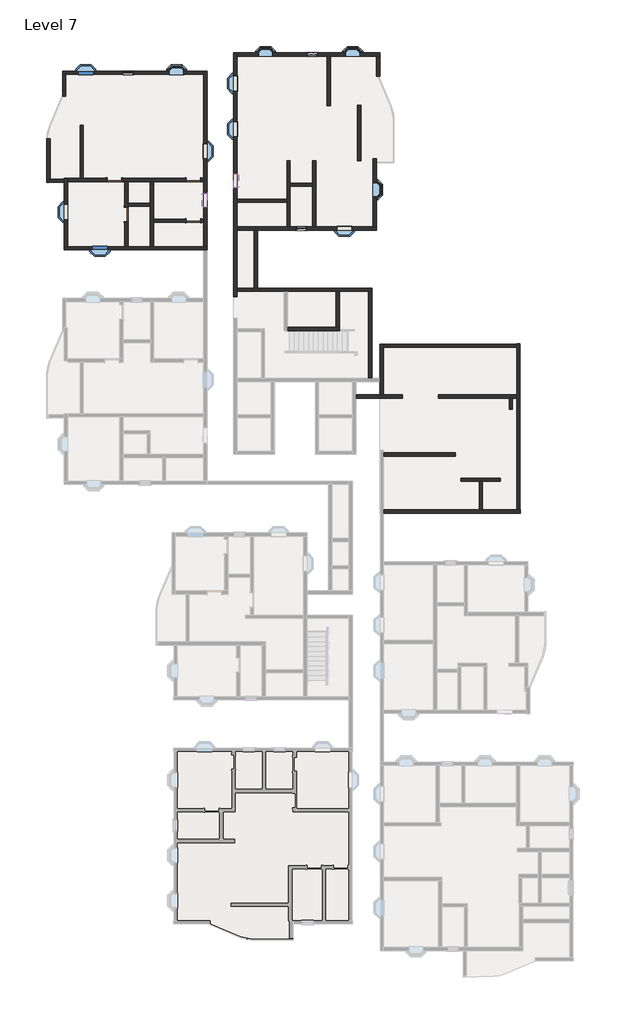
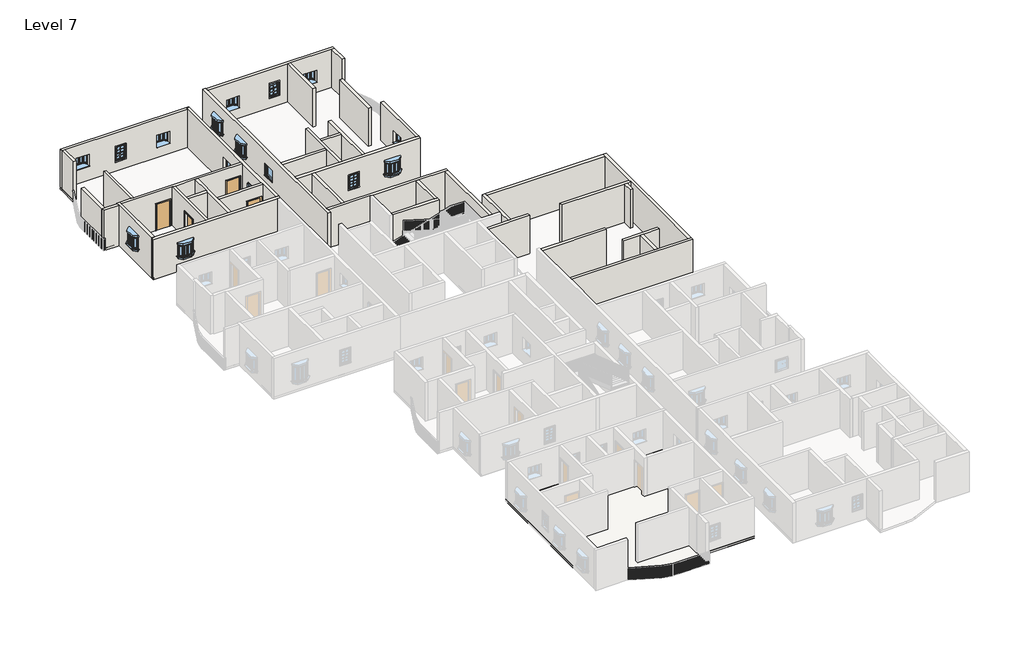
# One storey, part 4 of 14: 39 walls, 16 windows, 4 doors, 2 roofs.
"""IFC4 building model written with IfcOpenShell, lengths in millimetres."""

from ifc_helpers import new_model, si_unit, point, frame, frame_2d, origin, place, context, project, spatial, polyline, circle_curve, trimmed, segment, composite_curve, outline, extrude, faceted_brep, transform, mapped, element, save
from components import door_719f80de, window_910x910mm_67ef725a, window_8debb0fa, windows_sgl_w_glazing_bars_910x910mm_256712d0

model = new_model("IFC4")

# Units and contexts
model_context = context("Model", 3, world=origin())
ifc_project = project(units=[si_unit("LENGTHUNIT", "METRE", prefix="MILLI")], contexts=[model_context])

# Site, building, storey
site = spatial("IfcSite", under=ifc_project)
building = spatial("IfcBuilding", under=site)
storey = spatial("IfcBuildingStorey", under=building, Name="Level 7", Elevation=18288.0)

# Doors
placement = place(None, origin())
door_shape = door_719f80de(model_context)
element("IfcDoor", 1, ObjectType="Single-Flush : 36\" x 84\"", at=placement, inside=storey, context=model_context, shape_type="MappedRepresentation", body=[
    mapped(door_shape, transform((-16068.1391351, 22048.4083494, 18288.0), x_axis=(1.0, 0.0, 0.0), y_axis=(0.0, 1.0, 0.0), z_axis=(0.0, 0.0, 1.0))),
])
element("IfcDoor", 2, ObjectType="Single-Flush : 36\" x 84\"", at=placement, inside=storey, context=model_context, shape_type="MappedRepresentation", body=[
    mapped(door_shape, transform((-15306.1391351, 19864.0083494, 18288.0), x_axis=(0.0, 1.0, 0.0), y_axis=(-1.0, 0.0, 0.0), z_axis=(0.0, 0.0, 1.0))),
])
element("IfcDoor", 3, ObjectType="Single-Flush : 36\" x 84\"", at=placement, inside=storey, context=model_context, shape_type="MappedRepresentation", body=[
    mapped(door_shape, transform((-11057.9891351, 19470.3083494, 18288.0), x_axis=(1.0, 0.0, 0.0), y_axis=(0.0, 1.0, 0.0), z_axis=(0.0, 0.0, 1.0))),
])
element("IfcDoor", 4, ObjectType="Single-Flush : 36\" x 84\"", at=placement, inside=storey, context=model_context, shape_type="MappedRepresentation", body=[
    mapped(door_shape, transform((-11057.9891351, 22048.4083494, 18288.0), x_axis=(1.0, 0.0, 0.0), y_axis=(0.0, 1.0, 0.0), z_axis=(0.0, 0.0, 1.0))),
])

# Roofs
element("IfcRoof", 5, ObjectType="Generic - 12\"", at=placement, inside=storey, context=model_context, shape_type="SweptSolid", body=[
    extrude(outline(composite_curve([segment(polyline([(-10024.8708389, -25100.3416506), (-12290.487215, -25100.3416506), (-12290.487215, -13962.4416506), (-986.8891351, -13962.4416506), (-986.8891351, -25100.3416506), (-4746.0891351, -25100.3416506), (-4746.0891351, -26090.9416506), (-7315.6413127, -26090.9416506)]), True, "CONTINUOUS"), segment(trimmed(circle_curve(frame_2d((-7315.6413127, -24160.5416506)), 1930.4), [point((-7315.6413127, -26090.9416506))], [point((-8075.5356374, -25935.0851906))], False, "CARTESIAN"), True, "CONTINUOUS"), segment(polyline([(-8075.5356374, -25935.0851906), (-10024.8708389, -25100.3416506)]), True, "CONTINUOUS")], self_intersect=False)), frame((0.0, 0.0, 18288.0), z_axis=(0.0, 0.0, 1.0), x_axis=(1.0, 0.0, 0.0)), (0.0, 0.0, 1.0), 152.4),
])
element("IfcRoof", 6, ObjectType="Generic - 12\"", at=placement, inside=storey, context=model_context, shape_type="SweptSolid", body=[
    extrude(outline(composite_curve([segment(polyline([(-10024.8708389, -25100.3416506), (-12290.487215, -25100.3416506), (-12290.487215, -13962.4416506), (-986.8891351, -13962.4416506), (-986.8891351, -25100.3416506), (-4746.0891351, -25100.3416506), (-4746.0891351, -26090.9416506), (-7315.6413127, -26090.9416506)]), True, "CONTINUOUS"), segment(trimmed(circle_curve(frame_2d((-7315.6413127, -24160.5416506)), 1930.4), [point((-7315.6413127, -26090.9416506))], [point((-8075.5356374, -25935.0851906))], False, "CARTESIAN"), True, "CONTINUOUS"), segment(polyline([(-8075.5356374, -25935.0851906), (-10024.8708389, -25100.3416506)]), True, "CONTINUOUS")], self_intersect=False)), frame((0.0, 0.0, 18288.0), z_axis=(0.0, 0.0, 1.0), x_axis=(1.0, 0.0, 0.0)), (0.0, 0.0, 1.0), 152.4),
])

# Walls
element("IfcWall", 7, ObjectType="4.5\" p", at=placement, inside=storey, context=model_context, shape_type="Brep", body=[
    faceted_brep([(-10600.7891351, 21946.8083494, 20421.6), (-10600.7891351, 21946.8083494, 18288.0), (-10397.5891351, 21946.8083494, 18288.0), (-10397.5891351, 21946.8083494, 21336.0), (-13578.9391351, 21946.8083494, 21336.0), (-13782.1391351, 21946.8083494, 21336.0), (-15204.5391351, 21946.8083494, 21336.0), (-15407.7391351, 21946.8083494, 21336.0), (-19033.5891351, 21946.8083494, 21336.0), (-19033.5891351, 21946.8083494, 18288.0), (-16525.3391351, 21946.8083494, 18288.0), (-16525.3391351, 21946.8083494, 20421.6), (-15610.9391351, 21946.8083494, 20421.6), (-15610.9391351, 21946.8083494, 18288.0), (-15407.7391351, 21946.8083494, 18288.0), (-15204.5391351, 21946.8083494, 18288.0), (-13782.1391351, 21946.8083494, 18288.0), (-13578.9391351, 21946.8083494, 18288.0), (-11515.1891351, 21946.8083494, 18288.0), (-11515.1891351, 21946.8083494, 20421.6), (-10397.5891351, 22150.0083494, 18288.0), (-10600.7891351, 22150.0083494, 18288.0), (-10600.7891351, 22150.0083494, 20421.6), (-11515.1891351, 22150.0083494, 20421.6), (-11515.1891351, 22150.0083494, 18288.0), (-15610.9391351, 22150.0083494, 18288.0), (-15610.9391351, 22150.0083494, 20421.6), (-16525.3391351, 22150.0083494, 20421.6), (-16525.3391351, 22150.0083494, 18288.0), (-18042.9891351, 22150.0083494, 18288.0), (-18246.1891351, 22150.0083494, 18288.0), (-19033.5891351, 22150.0083494, 18288.0), (-19033.5891351, 22150.0083494, 21336.0), (-18246.1891351, 22150.0083494, 21336.0), (-18042.9891351, 22150.0083494, 21336.0), (-10397.5891351, 22150.0083494, 21336.0)], [[[0, 1, 2, 3, 4, 5, 6, 7, 8, 9, 10, 11, 12, 13, 14, 15, 16, 17, 18, 19]], [[20, 21, 22, 23, 24, 25, 26, 27, 28, 29, 30, 31, 32, 33, 34, 35]], [[10, 9, 31, 30, 29, 28]], [[2, 1, 21, 20]], [[18, 17, 16, 15, 14, 13, 25, 24]], [[8, 7, 6, 5, 4, 3, 35, 34, 33, 32]], [[9, 8, 32, 31]], [[3, 2, 20, 35]], [[26, 25, 13, 12]], [[27, 26, 12, 11]], [[28, 27, 11, 10]], [[22, 21, 1, 0]], [[23, 22, 0, 19]], [[24, 23, 19, 18]]]),
])
element("IfcWall", 8, ObjectType="4.5\" p", at=placement, inside=storey, context=model_context, shape_type="Brep", body=[
    faceted_brep([(-15407.7391351, 21946.8083494, 18288.0), (-15407.7391351, 20321.2083494, 18288.0), (-15407.7391351, 20321.2083494, 20421.6), (-15407.7391351, 19406.8083494, 20421.6), (-15407.7391351, 19406.8083494, 18288.0), (-15407.7391351, 17812.9583494, 18288.0), (-15407.7391351, 17812.9583494, 21336.0), (-15407.7391351, 21946.8083494, 21336.0), (-15204.5391351, 20321.2083494, 20421.6), (-15204.5391351, 20321.2083494, 18288.0), (-15204.5391351, 20372.0083494, 18288.0), (-15204.5391351, 20575.2083494, 18288.0), (-15204.5391351, 21946.8083494, 18288.0), (-15204.5391351, 21946.8083494, 21336.0), (-15204.5391351, 20575.2083494, 21336.0), (-15204.5391351, 20372.0083494, 21336.0), (-15204.5391351, 17812.9583494, 21336.0), (-15204.5391351, 17812.9583494, 18288.0), (-15204.5391351, 19406.8083494, 18288.0), (-15204.5391351, 19406.8083494, 20421.6)], [[[0, 1, 2, 3, 4, 5, 6, 7]], [[8, 9, 10, 11, 12, 13, 14, 15, 16, 17, 18, 19]], [[18, 17, 5, 4]], [[12, 11, 10, 9, 1, 0]], [[7, 6, 16, 15, 14, 13]], [[6, 5, 17, 16]], [[0, 7, 13, 12]], [[2, 1, 9, 8]], [[3, 2, 8, 19]], [[4, 3, 19, 18]]]),
])
element("IfcWall", 9, ObjectType="4.5\" p", at=placement, inside=storey, context=model_context, shape_type="Brep", body=[
    faceted_brep([(-13782.1391351, 21946.8083494, 18288.0), (-13782.1391351, 20575.2083494, 18288.0), (-13782.1391351, 20372.0083494, 18288.0), (-13782.1391351, 17812.9583494, 18288.0), (-13782.1391351, 17812.9583494, 21336.0), (-13782.1391351, 20372.0083494, 21336.0), (-13782.1391351, 20575.2083494, 21336.0), (-13782.1391351, 21946.8083494, 21336.0), (-13578.9391351, 21946.8083494, 18288.0), (-13578.9391351, 21946.8083494, 21336.0), (-13578.9391351, 19571.9083494, 21336.0), (-13578.9391351, 19368.7083494, 21336.0), (-13578.9391351, 17812.9583494, 21336.0), (-13578.9391351, 17812.9583494, 18288.0), (-13578.9391351, 19368.7083494, 18288.0), (-13578.9391351, 19571.9083494, 18288.0)], [[[0, 1, 2, 3, 4, 5, 6, 7]], [[8, 9, 10, 11, 12, 13, 14, 15]], [[3, 2, 1, 0, 8, 15, 14, 13]], [[7, 6, 5, 4, 12, 11, 10, 9]], [[4, 3, 13, 12]], [[0, 7, 9, 8]]]),
])
element("IfcWall", 10, ObjectType="4.5\" p", at=placement, inside=storey, context=model_context, shape_type="SweptSolid", body=[
    extrude(outline(polyline([(-13782.1391351, 20372.0083494), (-15204.5391351, 20372.0083494), (-15204.5391351, 20575.2083494), (-13782.1391351, 20575.2083494), (-13782.1391351, 20372.0083494)])), frame((0.0, 0.0, 18288.0), z_axis=(0.0, 0.0, 1.0), x_axis=(1.0, 0.0, 0.0)), (0.0, 0.0, 1.0), 3048.0),
])
element("IfcWall", 11, ObjectType="4.5\" p", at=placement, inside=storey, context=model_context, shape_type="SweptSolid", body=[
    extrude(outline(polyline([(20421.6, -10600.7891351), (18288.0, -10600.7891351), (18288.0, -10397.5891351), (21336.0, -10397.5891351), (21336.0, -13578.9391351), (18288.0, -13578.9391351), (18288.0, -11515.1891351), (20421.6, -11515.1891351), (20421.6, -10600.7891351)])), frame((0.0, 19368.7083494, 0.0), z_axis=(0.0, 1.0, 0.0), x_axis=(0.0, 0.0, 1.0)), (0.0, 0.0, 1.0), 203.2),
])
element("IfcWall", 12, ObjectType="4.5\" p", at=placement, inside=storey, context=model_context, shape_type="SweptSolid", body=[
    extrude(outline(polyline([(-18246.1891351, 22150.0083494), (-18246.1891351, 25515.5083494), (-18042.9891351, 25515.5083494), (-18042.9891351, 22150.0083494), (-18246.1891351, 22150.0083494)])), frame((0.0, 0.0, 18288.0), z_axis=(0.0, 0.0, 1.0), x_axis=(1.0, 0.0, 0.0)), (0.0, 0.0, 1.0), 3048.0),
])
element("IfcWall", 13, ObjectType="4.5\" p", at=placement, inside=storey, context=model_context, shape_type="SweptSolid", body=[
    extrude(outline(polyline([(-6993.9891351, 18875.1215905), (-6993.9891351, 15192.1215905), (-7197.1891351, 15192.1215905), (-7197.1891351, 18875.1215905), (-6993.9891351, 18875.1215905)])), frame((0.0, 0.0, 18288.0), z_axis=(0.0, 0.0, 1.0), x_axis=(1.0, 0.0, 0.0)), (0.0, 0.0, 1.0), 3048.0),
])
element("IfcWall", 14, ObjectType="4.5\" p", at=placement, inside=storey, context=model_context, shape_type="Brep", body=[
    faceted_brep([(-8289.3891351, 18875.1215905, 18288.0), (-7197.1891351, 18875.1215905, 18288.0), (-6993.9891351, 18875.1215905, 18288.0), (562.5108649, 18875.1215905, 18288.0), (562.5108649, 18875.1215905, 21336.0), (-6993.9891351, 18875.1215905, 21336.0), (-7197.1891351, 18875.1215905, 21336.0), (-8289.3891351, 18875.1215905, 21336.0), (-1017.6641351, 18875.1215905, 20398.0), (-1017.6641351, 18875.1215905, 19488.0), (-1927.6641351, 18875.1215905, 19488.0), (-1927.6641351, 18875.1215905, 20398.0), (-3876.1391351, 18875.1215905, 20269.2), (-3876.1391351, 18875.1215905, 19202.4), (-4536.5391351, 18875.1215905, 19202.4), (-4536.5391351, 18875.1215905, 20269.2), (-8289.3891351, 19078.3215905, 18288.0), (-8289.3891351, 19078.3215905, 21336.0), (-5120.7391351, 19078.3215905, 21336.0), (-4917.5391351, 19078.3215905, 21336.0), (-3495.1391351, 19078.3215905, 21336.0), (-3291.9391351, 19078.3215905, 21336.0), (346.6108649, 19078.3215905, 21336.0), (549.8108649, 19078.3215905, 21336.0), (562.5108649, 19078.3215905, 21336.0), (562.5108649, 19078.3215905, 18288.0), (549.8108649, 19078.3215905, 18288.0), (346.6108649, 19078.3215905, 18288.0), (-3291.9391351, 19078.3215905, 18288.0), (-3495.1391351, 19078.3215905, 18288.0), (-4917.5391351, 19078.3215905, 18288.0), (-5120.7391351, 19078.3215905, 18288.0), (-1017.6641351, 19078.3215905, 20398.0), (-1927.6641351, 19078.3215905, 20398.0), (-1927.6641351, 19078.3215905, 19488.0), (-1017.6641351, 19078.3215905, 19488.0), (-3876.1391351, 19078.3215905, 20269.2), (-4536.5391351, 19078.3215905, 20269.2), (-4536.5391351, 19078.3215905, 19202.4), (-3876.1391351, 19078.3215905, 19202.4)], [[[0, 1, 2, 3, 4, 5, 6, 7], [8, 9, 10, 11], [12, 13, 14, 15]], [[16, 17, 18, 19, 20, 21, 22, 23, 24, 25, 26, 27, 28, 29, 30, 31], [32, 33, 34, 35], [36, 37, 38, 39]], [[3, 2, 1, 0, 16, 31, 30, 29, 28, 27, 26, 25]], [[4, 3, 25, 24]], [[7, 6, 5, 4, 24, 23, 22, 21, 20, 19, 18, 17]], [[0, 7, 17, 16]], [[9, 8, 32, 35]], [[10, 9, 35, 34]], [[11, 10, 34, 33]], [[8, 11, 33, 32]], [[13, 12, 36, 39]], [[14, 13, 39, 38]], [[15, 14, 38, 37]], [[12, 15, 37, 36]]]),
])
element("IfcWall", 15, ObjectType="4.5\" p", at=placement, inside=storey, context=model_context, shape_type="SweptSolid", body=[
    extrude(outline(polyline([(19078.3215905, 18288.0), (19078.3215905, 21336.0), (23396.3215905, 21336.0), (23396.3215905, 18288.0), (19078.3215905, 18288.0)]), holes=[polyline([(21882.8215905, 20112.4), (20972.8215905, 20112.4), (20972.8215905, 19202.4), (21882.8215905, 19202.4), (21882.8215905, 20112.4)])]), frame((346.6108649, 0.0, 0.0), z_axis=(1.0, 0.0, 0.0), x_axis=(0.0, 1.0, 0.0)), (0.0, 0.0, 1.0), 203.2),
])
element("IfcWall", 16, ObjectType="4.5\" p", at=placement, inside=storey, context=model_context, shape_type="SweptSolid", body=[
    extrude(outline(polyline([(-5120.7391351, 20634.0715905), (-8289.3891351, 20634.0715905), (-8289.3891351, 20837.2715905), (-5120.7391351, 20837.2715905), (-5120.7391351, 20634.0715905)])), frame((0.0, 0.0, 18288.0), z_axis=(0.0, 0.0, 1.0), x_axis=(1.0, 0.0, 0.0)), (0.0, 0.0, 1.0), 3048.0),
])
element("IfcWall", 17, ObjectType="4.5\" p", at=placement, inside=storey, context=model_context, shape_type="Brep", body=[
    faceted_brep([(-5120.7391351, 23256.6215905, 18288.0), (-5120.7391351, 20837.2715905, 18288.0), (-5120.7391351, 20634.0715905, 18288.0), (-5120.7391351, 19078.3215905, 18288.0), (-5120.7391351, 19078.3215905, 21336.0), (-5120.7391351, 20634.0715905, 21336.0), (-5120.7391351, 20837.2715905, 21336.0), (-5120.7391351, 23256.6215905, 21336.0), (-4917.5391351, 23256.6215905, 18288.0), (-4917.5391351, 23256.6215905, 21336.0), (-4917.5391351, 21853.2715905, 21336.0), (-4917.5391351, 21650.0715905, 21336.0), (-4917.5391351, 19078.3215905, 21336.0), (-4917.5391351, 19078.3215905, 18288.0), (-4917.5391351, 21650.0715905, 18288.0), (-4917.5391351, 21853.2715905, 18288.0)], [[[0, 1, 2, 3, 4, 5, 6, 7]], [[8, 9, 10, 11, 12, 13, 14, 15]], [[3, 2, 1, 0, 8, 15, 14, 13]], [[7, 6, 5, 4, 12, 11, 10, 9]], [[0, 7, 9, 8]], [[4, 3, 13, 12]]]),
])
element("IfcWall", 18, ObjectType="4.5\" p", at=placement, inside=storey, context=model_context, shape_type="Brep", body=[
    faceted_brep([(-3495.1391351, 23256.6215905, 18288.0), (-3495.1391351, 21853.2715905, 18288.0), (-3495.1391351, 21650.0715905, 18288.0), (-3495.1391351, 19078.3215905, 18288.0), (-3495.1391351, 19078.3215905, 21336.0), (-3495.1391351, 21650.0715905, 21336.0), (-3495.1391351, 21853.2715905, 21336.0), (-3495.1391351, 23256.6215905, 21336.0), (-3291.9391351, 23256.6215905, 18288.0), (-3291.9391351, 23256.6215905, 21336.0), (-3291.9391351, 19078.3215905, 21336.0), (-3291.9391351, 19078.3215905, 18288.0)], [[[0, 1, 2, 3, 4, 5, 6, 7]], [[8, 9, 10, 11]], [[3, 2, 1, 0, 8, 11]], [[7, 6, 5, 4, 10, 9]], [[0, 7, 9, 8]], [[4, 3, 11, 10]]]),
])
element("IfcWall", 19, ObjectType="4.5\" p", at=placement, inside=storey, context=model_context, shape_type="SweptSolid", body=[
    extrude(outline(polyline([(-3495.1391351, 21650.0715905), (-4917.5391351, 21650.0715905), (-4917.5391351, 21853.2715905), (-3495.1391351, 21853.2715905), (-3495.1391351, 21650.0715905)])), frame((0.0, 0.0, 18288.0), z_axis=(0.0, 0.0, 1.0), x_axis=(1.0, 0.0, 0.0)), (0.0, 0.0, 1.0), 3048.0),
])
element("IfcWall", 20, ObjectType="4.5\" p", at=placement, inside=storey, context=model_context, shape_type="SweptSolid", body=[
    extrude(outline(polyline([(-1799.6891351, 14988.9215905), (-1799.6891351, 12709.2715905), (-2002.8891351, 12709.2715905), (-2002.8891351, 14988.9215905), (-1799.6891351, 14988.9215905)])), frame((0.0, 0.0, 18288.0), z_axis=(0.0, 0.0, 1.0), x_axis=(1.0, 0.0, 0.0)), (0.0, 0.0, 1.0), 3048.0),
])
element("IfcWall", 21, ObjectType="4.5\" p", at=placement, inside=storey, context=model_context, shape_type="Brep", body=[
    faceted_brep([(-5095.3391351, 12506.0715905, 18288.0), (-1786.9891351, 12506.0715905, 18288.0), (-1786.9891351, 12506.0715905, 21336.0), (-5095.3391351, 12506.0715905, 21336.0), (-5095.3391351, 12709.2715905, 18288.0), (-5095.3391351, 12709.2715905, 21336.0), (-2002.8891351, 12709.2715905, 21336.0), (-1799.6891351, 12709.2715905, 21336.0), (-1786.9891351, 12709.2715905, 21336.0), (-1786.9891351, 12709.2715905, 18288.0), (-1799.6891351, 12709.2715905, 18288.0), (-2002.8891351, 12709.2715905, 18288.0)], [[[0, 1, 2, 3]], [[4, 5, 6, 7, 8, 9, 10, 11]], [[1, 0, 4, 11, 10, 9]], [[2, 1, 9, 8]], [[3, 2, 8, 7, 6, 5]], [[0, 3, 5, 4]]]),
])
element("IfcWall", 22, ObjectType="4.5\" p", at=placement, inside=storey, context=model_context, shape_type="Brep", body=[
    faceted_brep([(-745.5891351, 8223.6457306, 18288.0), (2209.4205024, 8223.6457306, 18288.0), (2209.4205024, 8223.6457306, 21336.0), (-745.5891351, 8223.6457306, 21336.0), (-745.5891351, 8426.8457306, 18288.0), (-745.5891351, 8426.8457306, 21336.0), (793.5880523, 8426.8457306, 21336.0), (996.7880523, 8426.8457306, 21336.0), (2209.4205024, 8426.8457306, 21336.0), (2209.4205024, 8426.8457306, 18288.0), (996.7880523, 8426.8457306, 18288.0), (793.5880523, 8426.8457306, 18288.0)], [[[0, 1, 2, 3]], [[4, 5, 6, 7, 8, 9, 10, 11]], [[1, 0, 4, 11, 10, 9]], [[2, 1, 9, 8]], [[3, 2, 8, 7, 6, 5]], [[0, 3, 5, 4]]]),
])
element("IfcWall", 23, ObjectType="4.5\" p", at=placement, inside=storey, context=model_context, shape_type="Brep", body=[
    faceted_brep([(996.7880523, 8426.8457306, 18288.0), (996.7880523, 11443.0957306, 18288.0), (996.7880523, 11646.2957306, 18288.0), (996.7880523, 11646.2957306, 21336.0), (996.7880523, 11443.0957306, 21336.0), (996.7880523, 8426.8457306, 21336.0), (793.5880523, 8426.8457306, 18288.0), (793.5880523, 8426.8457306, 21336.0), (793.5880523, 9275.2949943, 21336.0), (793.5880523, 9478.4949943, 21336.0), (793.5880523, 11646.2957306, 21336.0), (793.5880523, 11646.2957306, 18288.0), (793.5880523, 9478.4949943, 18288.0), (793.5880523, 9275.2949943, 18288.0)], [[[0, 1, 2, 3, 4, 5]], [[6, 7, 8, 9, 10, 11, 12, 13]], [[2, 1, 0, 6, 13, 12, 11]], [[5, 4, 3, 10, 9, 8, 7]], [[0, 5, 7, 6]], [[3, 2, 11, 10]]]),
])
element("IfcWall", 24, ObjectType="4.5\" p", at=placement, inside=storey, context=model_context, shape_type="Brep", body=[
    faceted_brep([(9461.3380523, 8426.8457306, 18288.0), (4492.3034266, 8426.8457306, 18288.0), (4492.3034266, 8426.8457306, 21336.0), (9461.3380523, 8426.8457306, 21336.0), (9461.3380523, 8223.6457306, 18288.0), (9461.3380523, 8223.6457306, 21336.0), (9181.9380523, 8223.6457306, 21336.0), (8978.7380523, 8223.6457306, 21336.0), (4492.3034266, 8223.6457306, 21336.0), (4492.3034266, 8223.6457306, 18288.0), (8978.7380523, 8223.6457306, 18288.0), (9181.9380523, 8223.6457306, 18288.0)], [[[0, 1, 2, 3]], [[4, 5, 6, 7, 8, 9, 10, 11]], [[1, 0, 4, 11, 10, 9]], [[2, 1, 9, 8]], [[3, 2, 8, 7, 6, 5]], [[0, 3, 5, 4]]]),
])
element("IfcWall", 25, ObjectType="4.5\" p", at=placement, inside=storey, context=model_context, shape_type="Brep", body=[
    faceted_brep([(1007.0108649, 940.1957306, 18288.0), (9677.2380523, 940.1957306, 18288.0), (9677.2380523, 940.1957306, 21336.0), (1007.0108649, 940.1957306, 21336.0), (1007.0108649, 1143.3957306, 18288.0), (1007.0108649, 1143.3957306, 21336.0), (7073.7380523, 1143.3957306, 21336.0), (7276.9380523, 1143.3957306, 21336.0), (9461.3380523, 1143.3957306, 21336.0), (9664.5380523, 1143.3957306, 21336.0), (9677.2380523, 1143.3957306, 21336.0), (9677.2380523, 1143.3957306, 18288.0), (9664.5380523, 1143.3957306, 18288.0), (9461.3380523, 1143.3957306, 18288.0), (7276.9380523, 1143.3957306, 18288.0), (7073.7380523, 1143.3957306, 18288.0)], [[[0, 1, 2, 3]], [[4, 5, 6, 7, 8, 9, 10, 11, 12, 13, 14, 15]], [[1, 0, 4, 15, 14, 13, 12, 11]], [[2, 1, 11, 10]], [[3, 2, 10, 9, 8, 7, 6, 5]], [[0, 3, 5, 4]]]),
])
element("IfcWall", 26, ObjectType="4.5\" p", at=placement, inside=storey, context=model_context, shape_type="Brep", body=[
    faceted_brep([(9664.5380523, 1143.3957306, 18288.0), (9664.5380523, 11658.9957306, 18288.0), (9664.5380523, 11658.9957306, 21336.0), (9664.5380523, 1143.3957306, 21336.0), (9461.3380523, 1143.3957306, 18288.0), (9461.3380523, 1143.3957306, 21336.0), (9461.3380523, 8223.6457306, 21336.0), (9461.3380523, 8426.8457306, 21336.0), (9461.3380523, 11443.0957306, 21336.0), (9461.3380523, 11646.2957306, 21336.0), (9461.3380523, 11658.9957306, 21336.0), (9461.3380523, 11658.9957306, 18288.0), (9461.3380523, 11646.2957306, 18288.0), (9461.3380523, 11443.0957306, 18288.0), (9461.3380523, 8426.8457306, 18288.0), (9461.3380523, 8223.6457306, 18288.0)], [[[0, 1, 2, 3]], [[4, 5, 6, 7, 8, 9, 10, 11, 12, 13, 14, 15]], [[1, 0, 4, 15, 14, 13, 12, 11]], [[2, 1, 11, 10]], [[3, 2, 10, 9, 8, 7, 6, 5]], [[0, 3, 5, 4]]]),
])
element("IfcWall", 27, ObjectType="4.5\" p", at=placement, inside=storey, context=model_context, shape_type="SweptSolid", body=[
    extrude(outline(polyline([(-643.9891351, 23256.6215905), (-643.9891351, 26780.8715905), (-440.7891351, 26780.8715905), (-440.7891351, 23256.6215905), (-643.9891351, 23256.6215905)])), frame((0.0, 0.0, 18288.0), z_axis=(0.0, 0.0, 1.0), x_axis=(1.0, 0.0, 0.0)), (0.0, 0.0, 1.0), 3048.0),
])
element("IfcWall", 28, ObjectType="4.5\" p", at=placement, inside=storey, context=model_context, shape_type="SweptSolid", body=[
    extrude(outline(polyline([(-2568.0391351, 26760.9286213), (-2568.0391351, 29898.7215905), (-2364.8391351, 29898.7215905), (-2364.8391351, 26760.9286213), (-2568.0391351, 26760.9286213)])), frame((0.0, 0.0, 18288.0), z_axis=(0.0, 0.0, 1.0), x_axis=(1.0, 0.0, 0.0)), (0.0, 0.0, 1.0), 3048.0),
])
element("IfcWall", 29, ObjectType="4.5\" p", at=placement, inside=storey, context=model_context, shape_type="SweptSolid", body=[
    extrude(outline(polyline([(765.7108649, 29898.7215905), (765.7108649, 28631.1875845), (562.5108649, 28631.1875845), (562.5108649, 29898.7215905), (765.7108649, 29898.7215905)])), frame((0.0, 0.0, 18288.0), z_axis=(0.0, 0.0, 1.0), x_axis=(1.0, 0.0, 0.0)), (0.0, 0.0, 1.0), 3048.0),
])
element("IfcWall", 30, ObjectType="9\" w", at=placement, inside=storey, context=model_context, shape_type="Brep", body=[
    faceted_brep([(-10181.6891351, 17812.9583494, 18288.0), (-10194.3891351, 17812.9583494, 18288.0), (-10397.5891351, 17812.9583494, 18288.0), (-13578.9391351, 17812.9583494, 18288.0), (-13782.1391351, 17812.9583494, 18288.0), (-15204.5391351, 17812.9583494, 18288.0), (-15407.7391351, 17812.9583494, 18288.0), (-19033.5891351, 17812.9583494, 18288.0), (-19236.7891351, 17812.9583494, 18288.0), (-19249.4891351, 17812.9583494, 18288.0), (-19249.4891351, 17812.9583494, 21336.0), (-19236.7891351, 17812.9583494, 21336.0), (-19033.5891351, 17812.9583494, 21336.0), (-15407.7391351, 17812.9583494, 21336.0), (-15204.5391351, 17812.9583494, 21336.0), (-13782.1391351, 17812.9583494, 21336.0), (-13578.9391351, 17812.9583494, 21336.0), (-10397.5891351, 17812.9583494, 21336.0), (-10194.3891351, 17812.9583494, 21336.0), (-10181.6891351, 17812.9583494, 21336.0), (-16527.5391351, 17812.9583494, 20398.0), (-17437.5391351, 17812.9583494, 20398.0), (-17437.5391351, 17812.9583494, 19488.0), (-16527.5391351, 17812.9583494, 19488.0), (-10181.6891351, 17609.7583494, 18288.0), (-10181.6891351, 17609.7583494, 21336.0), (-19249.4891351, 17609.7583494, 21336.0), (-19249.4891351, 17609.7583494, 18288.0), (-16527.5391351, 17609.7583494, 20398.0), (-16527.5391351, 17609.7583494, 19488.0), (-17437.5391351, 17609.7583494, 19488.0), (-17437.5391351, 17609.7583494, 20398.0)], [[[0, 1, 2, 3, 4, 5, 6, 7, 8, 9, 10, 11, 12, 13, 14, 15, 16, 17, 18, 19], [20, 21, 22, 23]], [[24, 25, 26, 27], [28, 29, 30, 31]], [[9, 8, 7, 6, 5, 4, 3, 2, 1, 0, 24, 27]], [[10, 9, 27, 26]], [[19, 18, 17, 16, 15, 14, 13, 12, 11, 10, 26, 25]], [[0, 19, 25, 24]], [[29, 28, 20, 23]], [[30, 29, 23, 22]], [[31, 30, 22, 21]], [[28, 31, 21, 20]]]),
])
element("IfcWall", 31, ObjectType="9\" w", at=placement, inside=storey, context=model_context, shape_type="Brep", body=[
    faceted_brep([(-19033.5891351, 17812.9583494, 18288.0), (-19033.5891351, 21946.8083494, 18288.0), (-19033.5891351, 22150.0083494, 18288.0), (-19033.5891351, 22150.0083494, 21336.0), (-19033.5891351, 21946.8083494, 21336.0), (-19033.5891351, 17812.9583494, 21336.0), (-19033.5891351, 19555.0583494, 20398.0), (-19033.5891351, 20465.0583494, 20398.0), (-19033.5891351, 20465.0583494, 19488.0), (-19033.5891351, 19555.0583494, 19488.0), (-19236.7891351, 17812.9583494, 18288.0), (-19236.7891351, 17812.9583494, 21336.0), (-19236.7891351, 21889.6583494, 21336.0), (-19236.7891351, 22092.8583494, 21336.0), (-19236.7891351, 22150.0083494, 21336.0), (-19236.7891351, 22150.0083494, 18288.0), (-19236.7891351, 22092.8583494, 18288.0), (-19236.7891351, 21889.6583494, 18288.0), (-19236.7891351, 19555.0583494, 20398.0), (-19236.7891351, 19555.0583494, 19488.0), (-19236.7891351, 20465.0583494, 19488.0), (-19236.7891351, 20465.0583494, 20398.0)], [[[0, 1, 2, 3, 4, 5], [6, 7, 8, 9]], [[10, 11, 12, 13, 14, 15, 16, 17], [18, 19, 20, 21]], [[2, 1, 0, 10, 17, 16, 15]], [[5, 4, 3, 14, 13, 12, 11]], [[0, 5, 11, 10]], [[3, 2, 15, 14]], [[19, 18, 6, 9]], [[20, 19, 9, 8]], [[21, 20, 8, 7]], [[18, 21, 7, 6]]]),
])
element("IfcWall", 32, ObjectType="9\" w", at=placement, inside=storey, context=model_context, shape_type="Brep", body=[
    faceted_brep([(-10194.3891351, 17812.9583494, 18288.0), (-10194.3891351, 28849.2583494, 18288.0), (-10194.3891351, 28849.2583494, 21336.0), (-10194.3891351, 17812.9583494, 21336.0), (-10194.3891351, 24319.5083494, 20398.0), (-10194.3891351, 24319.5083494, 19488.0), (-10194.3891351, 23409.5083494, 19488.0), (-10194.3891351, 23409.5083494, 20398.0), (-10194.3891351, 20304.3583494, 20398.0), (-10194.3891351, 21214.3583494, 20398.0), (-10194.3891351, 21214.3583494, 19488.0), (-10194.3891351, 20304.3583494, 19488.0), (-10397.5891351, 17812.9583494, 18288.0), (-10397.5891351, 17812.9583494, 21336.0), (-10397.5891351, 19368.7083494, 21336.0), (-10397.5891351, 19571.9083494, 21336.0), (-10397.5891351, 21946.8083494, 21336.0), (-10397.5891351, 22150.0083494, 21336.0), (-10397.5891351, 28849.2583494, 21336.0), (-10397.5891351, 28849.2583494, 18288.0), (-10397.5891351, 22150.0083494, 18288.0), (-10397.5891351, 21946.8083494, 18288.0), (-10397.5891351, 19571.9083494, 18288.0), (-10397.5891351, 19368.7083494, 18288.0), (-10397.5891351, 24319.5083494, 20398.0), (-10397.5891351, 23409.5083494, 20398.0), (-10397.5891351, 23409.5083494, 19488.0), (-10397.5891351, 24319.5083494, 19488.0), (-10397.5891351, 20304.3583494, 20398.0), (-10397.5891351, 20304.3583494, 19488.0), (-10397.5891351, 21214.3583494, 19488.0), (-10397.5891351, 21214.3583494, 20398.0)], [[[0, 1, 2, 3], [4, 5, 6, 7], [8, 9, 10, 11]], [[12, 13, 14, 15, 16, 17, 18, 19, 20, 21, 22, 23], [24, 25, 26, 27], [28, 29, 30, 31]], [[1, 0, 12, 23, 22, 21, 20, 19]], [[2, 1, 19, 18]], [[3, 2, 18, 17, 16, 15, 14, 13]], [[0, 3, 13, 12]], [[5, 4, 24, 27]], [[6, 5, 27, 26]], [[7, 6, 26, 25]], [[4, 7, 25, 24]], [[29, 28, 8, 11]], [[30, 29, 11, 10]], [[31, 30, 10, 9]], [[28, 31, 9, 8]]]),
])
element("IfcWall", 33, ObjectType="9\" w", at=placement, inside=storey, context=model_context, shape_type="Brep", body=[
    faceted_brep([(-20341.6891351, 21889.6583494, 18288.0), (-19236.7891351, 21889.6583494, 18288.0), (-19236.7891351, 21889.6583494, 21336.0), (-20341.6891351, 21889.6583494, 21336.0), (-20341.6891351, 22092.8583494, 18288.0), (-20341.6891351, 22092.8583494, 21336.0), (-20138.4891351, 22092.8583494, 21336.0), (-19236.7891351, 22092.8583494, 21336.0), (-19236.7891351, 22092.8583494, 18288.0), (-20138.4891351, 22092.8583494, 18288.0)], [[[0, 1, 2, 3]], [[4, 5, 6, 7, 8, 9]], [[1, 0, 4, 9, 8]], [[3, 2, 7, 6, 5]], [[0, 3, 5, 4]], [[2, 1, 8, 7]]]),
])
element("IfcWall", 34, ObjectType="9\" w", at=placement, inside=storey, context=model_context, shape_type="SweptSolid", body=[
    extrude(outline(polyline([(-20341.6891351, 22092.8583494), (-20341.6891351, 24656.5948172), (-20138.4891351, 24656.5948172), (-20138.4891351, 22092.8583494), (-20341.6891351, 22092.8583494)])), frame((0.0, 0.0, 18288.0), z_axis=(0.0, 0.0, 1.0), x_axis=(1.0, 0.0, 0.0)), (0.0, 0.0, 1.0), 3048.0),
])
element("IfcWall", 35, ObjectType="9\" w", at=placement, inside=storey, context=model_context, shape_type="Brep", body=[
    faceted_brep([(-8492.5891351, 30114.6215905, 18288.0), (-8492.5891351, 14654.9471999, 18288.0), (-8492.5891351, 14654.9471999, 21336.0), (-8492.5891351, 30114.6215905, 21336.0), (-8492.5891351, 27703.9922564, 20398.0), (-8492.5891351, 27703.9922564, 19488.0), (-8492.5891351, 28613.9922564, 19488.0), (-8492.5891351, 28613.9922564, 20398.0), (-8492.5891351, 24808.3922564, 20398.0), (-8492.5891351, 24808.3922564, 19488.0), (-8492.5891351, 25718.3922564, 19488.0), (-8492.5891351, 25718.3922564, 20398.0), (-8492.5891351, 22451.1465905, 20398.0), (-8492.5891351, 21541.1465905, 20398.0), (-8492.5891351, 21541.1465905, 19488.0), (-8492.5891351, 22451.1465905, 19488.0), (-8289.3891351, 30114.6215905, 18288.0), (-8289.3891351, 30114.6215905, 21336.0), (-8289.3891351, 30101.9215905, 21336.0), (-8289.3891351, 29898.7215905, 21336.0), (-8289.3891351, 20837.2715905, 21336.0), (-8289.3891351, 20634.0715905, 21336.0), (-8289.3891351, 19078.3215905, 21336.0), (-8289.3891351, 18875.1215905, 21336.0), (-8289.3891351, 15192.1215905, 21336.0), (-8289.3891351, 14988.9215905, 21336.0), (-8289.3891351, 14654.9471999, 21336.0), (-8289.3891351, 14654.9471999, 18288.0), (-8289.3891351, 14988.9215905, 18288.0), (-8289.3891351, 15192.1215905, 18288.0), (-8289.3891351, 18875.1215905, 18288.0), (-8289.3891351, 19078.3215905, 18288.0), (-8289.3891351, 20634.0715905, 18288.0), (-8289.3891351, 20837.2715905, 18288.0), (-8289.3891351, 29898.7215905, 18288.0), (-8289.3891351, 30101.9215905, 18288.0), (-8289.3891351, 27703.9922564, 20398.0), (-8289.3891351, 28613.9922564, 20398.0), (-8289.3891351, 28613.9922564, 19488.0), (-8289.3891351, 27703.9922564, 19488.0), (-8289.3891351, 24808.3922564, 20398.0), (-8289.3891351, 25718.3922564, 20398.0), (-8289.3891351, 25718.3922564, 19488.0), (-8289.3891351, 24808.3922564, 19488.0), (-8289.3891351, 22451.1465905, 20398.0), (-8289.3891351, 22451.1465905, 19488.0), (-8289.3891351, 21541.1465905, 19488.0), (-8289.3891351, 21541.1465905, 20398.0)], [[[0, 1, 2, 3], [4, 5, 6, 7], [8, 9, 10, 11], [12, 13, 14, 15]], [[16, 17, 18, 19, 20, 21, 22, 23, 24, 25, 26, 27, 28, 29, 30, 31, 32, 33, 34, 35], [36, 37, 38, 39], [40, 41, 42, 43], [44, 45, 46, 47]], [[1, 0, 16, 35, 34, 33, 32, 31, 30, 29, 28, 27]], [[2, 1, 27, 26]], [[3, 2, 26, 25, 24, 23, 22, 21, 20, 19, 18, 17]], [[0, 3, 17, 16]], [[5, 4, 36, 39]], [[6, 5, 39, 38]], [[7, 6, 38, 37]], [[4, 7, 37, 36]], [[9, 8, 40, 43]], [[10, 9, 43, 42]], [[11, 10, 42, 41]], [[8, 11, 41, 40]], [[45, 44, 12, 15]], [[46, 45, 15, 14]], [[47, 46, 14, 13]], [[44, 47, 13, 12]]]),
])
element("IfcWall", 36, ObjectType="9\" w", at=placement, inside=storey, context=model_context, shape_type="Brep", body=[
    faceted_brep([(-8289.3891351, 14988.9215905, 18288.0), (-5298.5391351, 14988.9215905, 18288.0), (-5095.3391351, 14988.9215905, 18288.0), (-2002.8891351, 14988.9215905, 18288.0), (-1799.6891351, 14988.9215905, 18288.0), (54.5108649, 14988.9215905, 18288.0), (257.7108649, 14988.9215905, 18288.0), (270.4108649, 14988.9215905, 18288.0), (270.4108649, 14988.9215905, 21336.0), (257.7108649, 14988.9215905, 21336.0), (54.5108649, 14988.9215905, 21336.0), (-1799.6891351, 14988.9215905, 21336.0), (-2002.8891351, 14988.9215905, 21336.0), (-5095.3391351, 14988.9215905, 21336.0), (-5298.5391351, 14988.9215905, 21336.0), (-8289.3891351, 14988.9215905, 21336.0), (-8289.3891351, 15192.1215905, 18288.0), (-8289.3891351, 15192.1215905, 21336.0), (-7197.1891351, 15192.1215905, 21336.0), (-6993.9891351, 15192.1215905, 21336.0), (270.4108649, 15192.1215905, 21336.0), (270.4108649, 15192.1215905, 18288.0), (-6993.9891351, 15192.1215905, 18288.0), (-7197.1891351, 15192.1215905, 18288.0)], [[[0, 1, 2, 3, 4, 5, 6, 7, 8, 9, 10, 11, 12, 13, 14, 15]], [[16, 17, 18, 19, 20, 21, 22, 23]], [[7, 6, 5, 4, 3, 2, 1, 0, 16, 23, 22, 21]], [[8, 7, 21, 20]], [[15, 14, 13, 12, 11, 10, 9, 8, 20, 19, 18, 17]], [[0, 15, 17, 16]]]),
])
element("IfcWall", 37, ObjectType="9\" w", at=placement, inside=storey, context=model_context, shape_type="SweptSolid", body=[
    extrude(outline(polyline([(54.5108649, 9478.4949943), (54.5108649, 14988.9215905), (257.7108649, 14988.9215905), (257.7108649, 9478.4949943), (54.5108649, 9478.4949943)])), frame((0.0, 0.0, 18288.0), z_axis=(0.0, 0.0, 1.0), x_axis=(1.0, 0.0, 0.0)), (0.0, 0.0, 1.0), 3048.0),
])
element("IfcWall", 38, ObjectType="9\" w", at=placement, inside=storey, context=model_context, shape_type="SweptSolid", body=[
    extrude(outline(polyline([(9461.3380523, 11443.0957306), (996.7880523, 11443.0957306), (996.7880523, 11646.2957306), (9461.3380523, 11646.2957306), (9461.3380523, 11443.0957306)])), frame((0.0, 0.0, 18288.0), z_axis=(0.0, 0.0, 1.0), x_axis=(1.0, 0.0, 0.0)), (0.0, 0.0, 1.0), 3048.0),
])
element("IfcWall", 39, ObjectType="9\" w", at=placement, inside=storey, context=model_context, shape_type="SweptSolid", body=[
    extrude(outline(polyline([(8978.7380523, 7506.0957306), (8978.7380523, 8223.6457306), (9181.9380523, 8223.6457306), (9181.9380523, 7506.0957306), (8978.7380523, 7506.0957306)])), frame((0.0, 0.0, 18288.0), z_axis=(0.0, 0.0, 1.0), x_axis=(1.0, 0.0, 0.0)), (0.0, 0.0, 1.0), 3048.0),
])
element("IfcWall", 40, ObjectType="9\" w", at=placement, inside=storey, context=model_context, shape_type="SweptSolid", body=[
    extrude(outline(polyline([(7276.9380523, 2954.8622042), (7276.9380523, 1143.3957306), (7073.7380523, 1143.3957306), (7073.7380523, 2954.8622042), (7276.9380523, 2954.8622042)])), frame((0.0, 0.0, 18288.0), z_axis=(0.0, 0.0, 1.0), x_axis=(1.0, 0.0, 0.0)), (0.0, 0.0, 1.0), 3048.0),
])
element("IfcWall", 41, ObjectType="9\" w", at=placement, inside=storey, context=model_context, shape_type="Brep", body=[
    faceted_brep([(5904.1857655, 2954.8622042, 18288.0), (7073.7380523, 2954.8622042, 18288.0), (7276.9380523, 2954.8622042, 18288.0), (8418.7857655, 2954.8622042, 18288.0), (8418.7857655, 2954.8622042, 21336.0), (7276.9380523, 2954.8622042, 21336.0), (7073.7380523, 2954.8622042, 21336.0), (5904.1857655, 2954.8622042, 21336.0), (5904.1857655, 3158.0622042, 18288.0), (5904.1857655, 3158.0622042, 21336.0), (8418.7857655, 3158.0622042, 21336.0), (8418.7857655, 3158.0622042, 18288.0)], [[[0, 1, 2, 3, 4, 5, 6, 7]], [[8, 9, 10, 11]], [[3, 2, 1, 0, 8, 11]], [[4, 3, 11, 10]], [[7, 6, 5, 4, 10, 9]], [[0, 7, 9, 8]]]),
])
element("IfcWall", 42, ObjectType="9\" w", at=placement, inside=storey, context=model_context, shape_type="SweptSolid", body=[
    extrude(outline(polyline([(5571.3060189, 4550.8949943), (1007.0108649, 4550.8949943), (1007.0108649, 4754.0949943), (5571.3060189, 4754.0949943), (5571.3060189, 4550.8949943)])), frame((0.0, 0.0, 18288.0), z_axis=(0.0, 0.0, 1.0), x_axis=(1.0, 0.0, 0.0)), (0.0, 0.0, 1.0), 3048.0),
])
element("IfcWall", 43, ObjectType="9\" w", at=placement, inside=storey, context=model_context, shape_type="Brep", body=[
    faceted_brep([(-8289.3891351, 29898.7215905, 18288.0), (-2568.0391351, 29898.7215905, 18288.0), (-2364.8391351, 29898.7215905, 18288.0), (562.5108649, 29898.7215905, 18288.0), (765.7108649, 29898.7215905, 18288.0), (765.7108649, 29898.7215905, 21336.0), (562.5108649, 29898.7215905, 21336.0), (-2364.8391351, 29898.7215905, 21336.0), (-2568.0391351, 29898.7215905, 21336.0), (-8289.3891351, 29898.7215905, 21336.0), (-6931.4641351, 29898.7215905, 20112.4), (-6021.4641351, 29898.7215905, 20112.4), (-6021.4641351, 29898.7215905, 19202.4), (-6931.4641351, 29898.7215905, 19202.4), (-1406.9641351, 29898.7215905, 20112.4), (-496.9641351, 29898.7215905, 20112.4), (-496.9641351, 29898.7215905, 19202.4), (-1406.9641351, 29898.7215905, 19202.4), (-3844.3891351, 29898.7215905, 20269.2), (-3183.9891351, 29898.7215905, 20269.2), (-3183.9891351, 29898.7215905, 19202.4), (-3844.3891351, 29898.7215905, 19202.4), (-8289.3891351, 30101.9215905, 18288.0), (-8289.3891351, 30101.9215905, 21336.0), (765.7108649, 30101.9215905, 21336.0), (765.7108649, 30101.9215905, 18288.0), (-6931.4641351, 30101.9215905, 20112.4), (-6931.4641351, 30101.9215905, 19202.4), (-6021.4641351, 30101.9215905, 19202.4), (-6021.4641351, 30101.9215905, 20112.4), (-1406.9641351, 30101.9215905, 20112.4), (-1406.9641351, 30101.9215905, 19202.4), (-496.9641351, 30101.9215905, 19202.4), (-496.9641351, 30101.9215905, 20112.4), (-3844.3891351, 30101.9215905, 20269.2), (-3844.3891351, 30101.9215905, 19202.4), (-3183.9891351, 30101.9215905, 19202.4), (-3183.9891351, 30101.9215905, 20269.2)], [[[0, 1, 2, 3, 4, 5, 6, 7, 8, 9], [10, 11, 12, 13], [14, 15, 16, 17], [18, 19, 20, 21]], [[22, 23, 24, 25], [26, 27, 28, 29], [30, 31, 32, 33], [34, 35, 36, 37]], [[4, 3, 2, 1, 0, 22, 25]], [[9, 8, 7, 6, 5, 24, 23]], [[27, 26, 10, 13]], [[28, 27, 13, 12]], [[29, 28, 12, 11]], [[26, 29, 11, 10]], [[31, 30, 14, 17]], [[32, 31, 17, 16]], [[33, 32, 16, 15]], [[30, 33, 15, 14]], [[35, 34, 18, 21]], [[36, 35, 21, 20]], [[37, 36, 20, 19]], [[34, 37, 19, 18]], [[0, 9, 23, 22]], [[5, 4, 25, 24]]]),
])
element("IfcWall", 44, ObjectType="9\" w", at=placement, inside=storey, context=model_context, shape_type="Brep", body=[
    faceted_brep([(-19351.0891351, 28747.6583494, 18288.0), (-19147.8891351, 28747.6583494, 18288.0), (-10181.6891351, 28747.6583494, 18288.0), (-10181.6891351, 28747.6583494, 21336.0), (-19147.8891351, 28747.6583494, 21336.0), (-19351.0891351, 28747.6583494, 21336.0), (-18332.8891351, 28747.6583494, 20398.0), (-17422.8891351, 28747.6583494, 20398.0), (-17422.8891351, 28747.6583494, 19488.0), (-18332.8891351, 28747.6583494, 19488.0), (-12579.7891351, 28747.6583494, 20112.4), (-11669.7891351, 28747.6583494, 20112.4), (-11669.7891351, 28747.6583494, 19202.4), (-12579.7891351, 28747.6583494, 19202.4), (-14845.7641351, 28747.6583494, 20269.2), (-14845.7641351, 28747.6583494, 19202.4), (-15506.1641351, 28747.6583494, 19202.4), (-15506.1641351, 28747.6583494, 20269.2), (-19351.0891351, 28950.8583494, 18288.0), (-19351.0891351, 28950.8583494, 21336.0), (-10181.6891351, 28950.8583494, 21336.0), (-10181.6891351, 28950.8583494, 18288.0), (-18332.8891351, 28950.8583494, 20398.0), (-18332.8891351, 28950.8583494, 19488.0), (-17422.8891351, 28950.8583494, 19488.0), (-17422.8891351, 28950.8583494, 20398.0), (-12579.7891351, 28950.8583494, 20112.4), (-12579.7891351, 28950.8583494, 19202.4), (-11669.7891351, 28950.8583494, 19202.4), (-11669.7891351, 28950.8583494, 20112.4), (-14845.7641351, 28950.8583494, 20269.2), (-15506.1641351, 28950.8583494, 20269.2), (-15506.1641351, 28950.8583494, 19202.4), (-14845.7641351, 28950.8583494, 19202.4)], [[[0, 1, 2, 3, 4, 5], [6, 7, 8, 9], [10, 11, 12, 13], [14, 15, 16, 17]], [[18, 19, 20, 21], [22, 23, 24, 25], [26, 27, 28, 29], [30, 31, 32, 33]], [[2, 1, 0, 18, 21]], [[3, 2, 21, 20]], [[5, 4, 3, 20, 19]], [[23, 22, 6, 9]], [[24, 23, 9, 8]], [[25, 24, 8, 7]], [[22, 25, 7, 6]], [[27, 26, 10, 13]], [[28, 27, 13, 12]], [[29, 28, 12, 11]], [[26, 29, 11, 10]], [[15, 14, 30, 33]], [[16, 15, 33, 32]], [[17, 16, 32, 31]], [[14, 17, 31, 30]], [[0, 5, 19, 18]]]),
])
element("IfcWall", 45, ObjectType="9\" w", at=placement, inside=storey, context=model_context, shape_type="SweptSolid", body=[
    extrude(outline(polyline([(-19147.8891351, 28747.6583494), (-19147.8891351, 27344.9858981), (-19351.0891351, 27344.9858981), (-19351.0891351, 28747.6583494), (-19147.8891351, 28747.6583494)])), frame((0.0, 0.0, 18288.0), z_axis=(0.0, 0.0, 1.0), x_axis=(1.0, 0.0, 0.0)), (0.0, 0.0, 1.0), 3048.0),
])

# Windows
window_910x910mm_shape = window_910x910mm_67ef725a(model_context)
element("IfcWindow", 46, ObjectType="910x910mm", at=placement, inside=storey, context=model_context, shape_type="MappedRepresentation", body=[
    mapped(window_910x910mm_shape, transform((-10304.445703, 23294.5083494, 18288.0), x_axis=(0.0, -1.0, 0.0), y_axis=(1.0, 0.0, 0.0), z_axis=(0.0, 0.0, 1.0))),
])
element("IfcWindow", 47, ObjectType="910x910mm", at=placement, inside=storey, context=model_context, shape_type="MappedRepresentation", body=[
    mapped(window_910x910mm_shape, transform((-19126.7325673, 20580.0583494, 18288.0), x_axis=(0.0, 1.0, 0.0), y_axis=(-1.0, 0.0, 0.0), z_axis=(0.0, 0.0, 1.0))),
])
element("IfcWindow", 48, ObjectType="910x910mm", at=placement, inside=storey, context=model_context, shape_type="MappedRepresentation", body=[
    mapped(window_910x910mm_shape, transform((-17552.5391351, 17719.8149172, 18288.0), x_axis=(-1.0, 0.0, 0.0), y_axis=(0.0, -1.0, 0.0), z_axis=(0.0, 0.0, 1.0))),
])
element("IfcWindow", 49, ObjectType="910x910mm", at=placement, inside=storey, context=model_context, shape_type="MappedRepresentation", body=[
    mapped(window_910x910mm_shape, transform((-8382.5325673, 28728.9922564, 18288.0), x_axis=(0.0, 1.0, 0.0), y_axis=(-1.0, 0.0, 0.0), z_axis=(0.0, 0.0, 1.0))),
])
element("IfcWindow", 50, ObjectType="910x910mm", at=placement, inside=storey, context=model_context, shape_type="MappedRepresentation", body=[
    mapped(window_910x910mm_shape, transform((-8382.5325673, 25833.3922564, 18288.0), x_axis=(0.0, 1.0, 0.0), y_axis=(-1.0, 0.0, 0.0), z_axis=(0.0, 0.0, 1.0))),
])
element("IfcWindow", 51, ObjectType="910x910mm", at=placement, inside=storey, context=model_context, shape_type="MappedRepresentation", body=[
    mapped(window_910x910mm_shape, transform((-5906.4641351, 29991.8650227, 18002.4), x_axis=(1.0, 0.0, 0.0), y_axis=(0.0, 1.0, 0.0), z_axis=(0.0, 0.0, 1.0))),
])
element("IfcWindow", 52, ObjectType="910x910mm", at=placement, inside=storey, context=model_context, shape_type="MappedRepresentation", body=[
    mapped(window_910x910mm_shape, transform((-381.9641351, 29991.8650227, 18002.4), x_axis=(1.0, 0.0, 0.0), y_axis=(0.0, 1.0, 0.0), z_axis=(0.0, 0.0, 1.0))),
])
element("IfcWindow", 53, ObjectType="910x910mm", at=placement, inside=storey, context=model_context, shape_type="MappedRepresentation", body=[
    mapped(window_910x910mm_shape, transform((-17307.8891351, 28840.8017816, 18288.0), x_axis=(1.0, 0.0, 0.0), y_axis=(0.0, 1.0, 0.0), z_axis=(0.0, 0.0, 1.0))),
])
element("IfcWindow", 54, ObjectType="910x910mm", at=placement, inside=storey, context=model_context, shape_type="MappedRepresentation", body=[
    mapped(window_910x910mm_shape, transform((-11554.7891351, 28840.8017816, 18002.4), x_axis=(1.0, 0.0, 0.0), y_axis=(0.0, 1.0, 0.0), z_axis=(0.0, 0.0, 1.0))),
])
element("IfcWindow", 55, ObjectType="910x910mm", at=placement, inside=storey, context=model_context, shape_type="MappedRepresentation", body=[
    mapped(window_910x910mm_shape, transform((439.754297, 20857.8215905, 18002.4), x_axis=(0.0, -1.0, 0.0), y_axis=(1.0, 0.0, 0.0), z_axis=(0.0, 0.0, 1.0))),
])
element("IfcWindow", 56, ObjectType="910x910mm", at=placement, inside=storey, context=model_context, shape_type="MappedRepresentation", body=[
    mapped(window_910x910mm_shape, transform((-2042.6641351, 18985.1781583, 18288.0), x_axis=(-1.0, 0.0, 0.0), y_axis=(0.0, -1.0, 0.0), z_axis=(0.0, 0.0, 1.0))),
])
window_shape = window_8debb0fa(model_context)
element("IfcWindow", 57, ObjectType="Window-Double-Hung : 26\" x 42\"", at=placement, inside=storey, context=model_context, shape_type="MappedRepresentation", body=[
    mapped(window_shape, transform((-3514.1891351, 30000.3215905, 18288.0), x_axis=(1.0, 0.0, 0.0), y_axis=(0.0, 1.0, 0.0), z_axis=(0.0, 0.0, 1.0))),
])
element("IfcWindow", 58, ObjectType="Window-Double-Hung : 26\" x 42\"", at=placement, inside=storey, context=model_context, shape_type="MappedRepresentation", body=[
    mapped(window_shape, transform((-15175.9641351, 28849.2583494, 18288.0), x_axis=(-1.0, 0.0, 0.0), y_axis=(0.0, -1.0, 0.0), z_axis=(0.0, 0.0, 1.0))),
])
element("IfcWindow", 59, ObjectType="Window-Double-Hung : 26\" x 42\"", at=placement, inside=storey, context=model_context, shape_type="MappedRepresentation", body=[
    mapped(window_shape, transform((-4206.3391351, 18976.7215905, 18288.0), x_axis=(-1.0, 0.0, 0.0), y_axis=(0.0, -1.0, 0.0), z_axis=(0.0, 0.0, 1.0))),
])
windows_sgl_w_glazing_bars_910x910mm_shape = windows_sgl_w_glazing_bars_910x910mm_256712d0(model_context)
element("IfcWindow", 60, ObjectType="Windows_Sgl_w-Glazing_Bars : 910x910mm", at=placement, inside=storey, context=model_context, shape_type="MappedRepresentation", body=[
    mapped(windows_sgl_w_glazing_bars_910x910mm_shape, transform((-10287.5325673, 20759.3583494, 18288.0), x_axis=(0.0, 1.0, 0.0), y_axis=(-1.0, 0.0, 0.0), z_axis=(0.0, 0.0, 1.0))),
])
element("IfcWindow", 61, ObjectType="Windows_Sgl_w-Glazing_Bars : 910x910mm", at=placement, inside=storey, context=model_context, shape_type="MappedRepresentation", body=[
    mapped(windows_sgl_w_glazing_bars_910x910mm_shape, transform((-8399.445703, 21996.1465905, 18288.0), x_axis=(0.0, -1.0, 0.0), y_axis=(1.0, 0.0, 0.0), z_axis=(0.0, 0.0, 1.0))),
])

save(model, "model.ifc")

# Revit data of these elements
# Type "Single-Flush : 36\" x 84\""
#   Type Mark = "1"
#   Construction Type Id = "MDOOR"
#   Assembly Code = "C1020"
#   Analytic Construction = "Metal"
#   Thickness = 0' - 2"
#   Heat Transfer Coefficient (U) = 0.651978 BTU/(h·ft²·°F)
#   Height = 7' - 0"
#   Trim Projection Ext = 0' - 1"
#   Trim Projection Int = 0' - 1"
#   Trim Width = 0' - 3"
#   Width = 3' - 0"
#   Define Thermal Properties by = 1
#   Define Thermal Properties by = 1
#   Door Material = Door - Panel
#   Frame Material = Door - Frame
#   Visual Light Transmittance = 0
#   Solar Heat Gain Coefficient = 0
#   Function = (empty or 0)
#   Wall Closure = (empty or 0)
# Type "Generic - 12\""
#   Assembly Code = "B1020"
#   Layers, outside or top first: 0' - 6" no material (function 1)
# Type "4.5\" p"
#   Assembly Code = "B2010"
#   Layers, outside or top first: 0' - 8" no material (function 1)
# Type "9\" w"
#   Assembly Code = "B2010"
#   Layers, outside or top first: 0' - 8" no material (function 1)
# Type "910x910mm"
#   Type Mark = "18"
#   Operation = "UserDefined"
#   Construction Type Id = "GSP4R"
#   Keynote = "L10"
#   Analytic Construction = "1/8 in Pilkington single glazing"
#   Wrap Layers (Ext) from Ext = 0' - 4.03543"
#   Wrap Layers (Int) from Ext = 0' - 6.98819"
#   Window Board Projection = 0' - 0.98425"
#   Window Board Extention = 0' - 0.98425"
#   Visual Light Transmittance = 0.9
#   Solar Heat Gain Coefficient = 0.78
#   Heat Transfer Coefficient (U) = 0.6496 BTU/(h·ft²·°F)
#   Glazing Thickness = 0' - 0.94488"
#   DONT CHANGE - Splay Width = 0' - 7.41997"
#   Rough Width = 2' - 11.82677"
#   Rough Height = 2' - 11.82677"
#   Roof Thickness = 0' - 4.92126"
#   Roof Overhang = 0' - 1.5748"
#   Plinth Thickness = 0' - 6.88976"
#   Height = 2' - 11.82677"
#   Width = 2' - 11.82677"
#   Frame Depth = 0' - 2.55906"
#   Default Head Height = 6' - 11.07087"
#   Cill Depth = 0' - 3.44488"
#   Cavity Closer Width = 0' - 1.9685"
#   Cavity Closer Offset from Ext = 0' - 4.03543"
#   Cavity Closer Depth = 0' - 3.34646"
#   Vis - Cavity Closers = yes
#   Define Thermal Properties by = 1
#   Material Trim = Window Frame
#   Material Glass = Glass
#   Material Frame = Window Frame
#   Manufacturer = ""
#   Wall Closure = (empty or 0)
# Type "Window-Double-Hung : 26\" x 42\""
#   Type Mark = "11"
#   Fire Rating = "0.5h"
#   Construction Type Id = "DG-DR"
#   Assembly Code = "B2020100"
#   Analytic Construction = "Double glazing - domestic"
#   Wall Thickness [instance default] = 0' - 6"
#   Window Inset [instance default] = 0' - 0"
#   Visual Light Transmittance = 0.81
#   Thermal Resistance (R) = 1.8146 (h·ft²·°F)/BTU
#   Solar Heat Gain Coefficient = 0.76
#   Muntin Width = 1' - 8"
#   Muntin Height = 1' - 5 1/8"
#   Interior Wall Closure [instance default] = 0' - 1 1/2"
#   Rough Width = 2' - 2 1/2"
#   Rough Height = 3' - 6 1/2"
#   Frame Extension [instance default] = 0' - 1 1/4"
#   Exterior Wall Closure [instance default] = 0' - 0 1/2"
#   Extension Jamb [instance default] = 0' - 1 1/2"
#   Heat Transfer Coefficient (U) = 0.5511 BTU/(h·ft²·°F)
#   Height = 3' - 6"
#   Width = 2' - 2"
#   Define Thermal Properties by = 1
#   Top Muntin Visibility = yes
#   Indicator Visibility [instance default] = yes
#   Extension Jamb Visibility [instance default] = yes
#   Interior Trim Visibility [instance default] = yes
#   Exterior Trim Visibility [instance default] = yes
#   Define Thermal Properties by = 1
#   Bottom Muntin Visibility = yes
#   Muntin Pattern = Muntin Pattern_2x2 : Muntin Pattern_2x2
#   Interior Trim Material = Wood - Stained
#   Interior Trim = Trim-Window-Interior-Flat : Picture Frame
#   Exterior Trim Material = Clad - White
#   Exterior Trim = Trim-Window-Exterior-Flat : with Sill
#   Glass Panel Material = Glass
#   Exterior Frame Material = Clad - White
#   Interior Frame Material = Wood - Stained
#   Wall Closure = (empty or 0)
# Type "Windows_Sgl_w-Glazing_Bars : 910x910mm"
#   Type Mark = "24"
#   Operation = "SinglePanel"
#   Construction Type Id = "SGL"
#   Manufacturer = "Revit"
#   Keynote = "L10"
#   Analytic Construction = "Large single-glazed windows"
#   Wrap Layers (Ext) from Ext = 0' - 4.03543"
#   Wrap Layers (Int) from Ext = 0' - 6.98819"
#   Window Board Projection = 0' - 0.98425"
#   Window Board Extension = 0' - 0.98425"
#   Visual Light Transmittance = 0.9
#   Solar Heat Gain Coefficient = 0.86
#   Rough Width = 2' - 11.82677"
#   Rough Height = 2' - 11.82677"
#   Height = 2' - 11.82677"
#   Width = 2' - 11.82677"
#   Heat Transfer Coefficient (U) = 0.979472 BTU/(h·ft²·°F)
#   Glazing Thickness = 0' - 0.94488"
#   Glazing Bar Thickness = 0' - 0.7874"
#   FrameOffset - External = 0' - 3.14961"
#   Frame Depth = 0' - 2.55906"
#   Default Head Height = 6' - 11.07087"
#   Cill Depth = 0' - 3.44488"
#   Cavity Closer Width = 0' - 1.9685"
#   Cavity Closer Offset from Ext = 0' - 4.03543"
#   Cavity Closer Depth = 0' - 3.34646"
#   Vis - Glazing Bars = yes
#   Vis - Cavity Closers = yes
#   Define Thermal Properties by = 1
#   Material Trim = Window Frame
#   Material Glazing Bars = Window Frame
#   Material Glass = Glass
#   Material Frame = Window Frame
#   Wall Closure = (empty or 0)
# Elements 1, 2, 3, 4 (IfcDoor, "Single-Flush : 36\" x 84\"")
#   Phase Created = New Construction
#   Materials on its faces: "Door - Frame", "Door - Panel"
# Element 5 (IfcRoof, "Generic - 12\"")
#   built-in parameter 1001705 = 60.5 (stored number, unit not read)
#   built-in parameter 1001710 = 33615
#   Phase Created = New Construction
#   Materials on its faces: "Default Roof"
# Element 6 (IfcRoof, "Generic - 12\"")
#   built-in parameter 1001705 = 60.5 (stored number, unit not read)
#   built-in parameter 1001710 = 33615
#   Phase Created = New Construction
#   Materials on its faces: "Default Roof", "Carpet (1)"
# Elements 7, 8, 9, 10, 11, 16, 17, 18, 19, 20, 21, 22, 24 (IfcWall, "4.5\" p")
#   Top Offset = 0' - 0"
#   Base Offset = 0' - 0"
#   wall height = 10' - 0"
#   Phase Created = New Construction
#   Base Constraint = Level 7
#   Top Constraint = Level 8
#   Materials on its faces: "Default Wall"
# Element 12 (IfcWall, "4.5\" p")
#   Top Offset = 0' - 0"
#   Base Offset = 0' - 0"
#   wall height = 10' - 0"
#   Phase Created = New Construction
#   Base Constraint = Level 7
#   Top Constraint = Level 8
#   Materials on its faces: "Default Wall", "Grass"
# Element 13 (IfcWall, "4.5\" p")
#   Top Offset = 0' - 0"
#   Base Offset = 0' - 0"
#   wall height = 10' - 0"
#   Phase Created = New Construction
#   Base Constraint = Level 7
#   Top Constraint = Level 8
#   Materials on its faces: "Default Wall", "Wood - Stained"
# Elements 14, 15 (IfcWall, "4.5\" p")
#   Top Offset = 0' - 0"
#   Base Offset = 0' - 0"
#   wall height = 10' - 0"
#   Phase Created = New Construction
#   Base Constraint = Level 7
#   Top Constraint = Level 8
#   Materials on its faces: "Default Wall", "Parking Stripe"
# Elements 23, 26 (IfcWall, "4.5\" p")
#   Top Offset = 0' - 0"
#   Base Offset = 0' - 0"
#   wall height = 10' - 0"
#   Phase Created = New Construction
#   Base Constraint = Level 7
#   Top Constraint = Level 8
#   Materials on its faces: "Default Wall", "Window Frame"
# Element 25 (IfcWall, "4.5\" p")
#   Top Offset = 0' - 0"
#   Base Offset = 0' - 0"
#   wall height = 10' - 0"
#   Phase Created = New Construction
#   Base Constraint = Level 7
#   Top Constraint = Level 8
#   Materials on its faces: "Default Wall", "Carpet (1)"
# Elements 27, 28 (IfcWall, "4.5\" p")
#   Top Offset = 0' - 0"
#   Base Offset = 0' - 0"
#   Unconnected Height = 10' - 0"
#   wall height = 10' - 0"
#   Phase Created = New Construction
#   Base Constraint = Level 7
#   Materials on its faces: "Default Wall", "Brick, Soldier Course"
# Element 29 (IfcWall, "4.5\" p")
#   Top Offset = 0' - 0"
#   Base Offset = 0' - 0"
#   Unconnected Height = 10' - 0"
#   wall height = 10' - 0"
#   Phase Created = New Construction
#   Base Constraint = Level 7
#   Materials on its faces: "Default Wall", "Default Mass Interior Wall"
# Elements 30, 39, 40, 41, 42 (IfcWall, "9\" w")
#   Top Offset = 0' - 0"
#   Base Offset = 0' - 0"
#   wall height = 10' - 0"
#   Phase Created = New Construction
#   Base Constraint = Level 7
#   Top Constraint = Level 8
#   Materials on its faces: "Default Wall"
# Elements 31, 45 (IfcWall, "9\" w")
#   Top Offset = 0' - 0"
#   Base Offset = 0' - 0"
